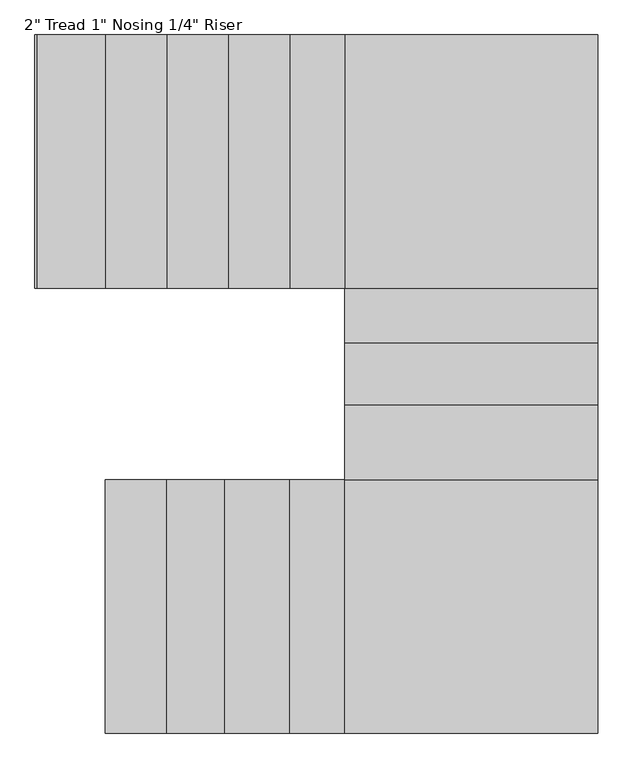
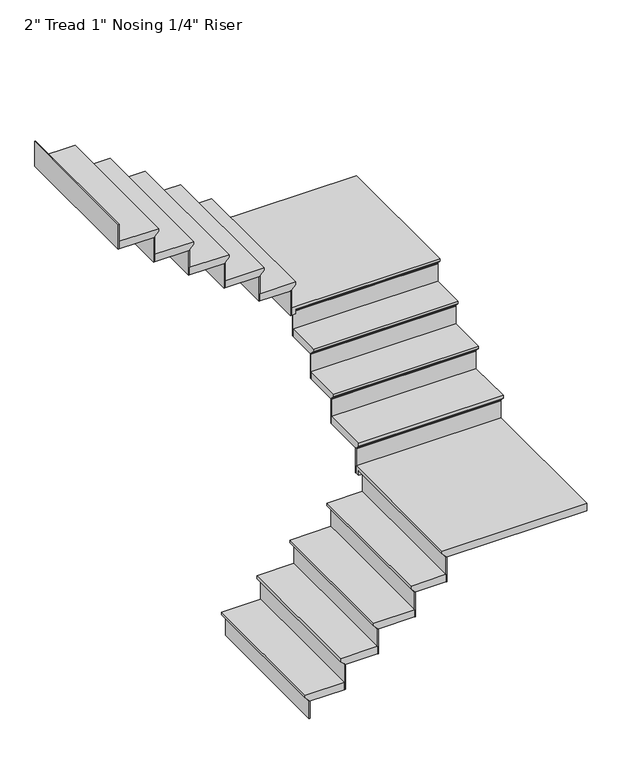
"""IFC4 building model written with IfcOpenShell, lengths in millimetres: stair flight geometry."""

from ifc_helpers import new_model, si_unit, origin, place, context, project, spatial, faceted_brep, source, transform, mapped, element, save


def stair_flight_c017ec09(model_context):
    return source(origin(), model_context, "Body", "Brep", [
        faceted_brep([(344.764115, -6141.1350571, 12951.8833333), (344.764115, -6141.1350571, 12970.9333333), (344.764115, -5201.3350571, 12970.9333333), (344.764115, -5201.3350571, 12951.8833333), (370.164115, -6141.1350571, 12926.4833333), (370.164115, -5201.3350571, 12926.4833333), (598.764115, -6141.1350571, 12970.9333333), (598.764115, -5201.3350571, 12970.9333333), (370.164115, -5201.3350571, 12920.1333333), (598.764115, -5201.3350571, 12920.1333333), (598.764115, -6141.1350571, 12920.1333333), (370.164115, -6141.1350571, 12920.1333333)], [[[0, 1, 2, 3]], [[4, 0, 3, 5]], [[2, 1, 6, 7]], [[8, 9, 10, 11]], [[2, 7, 9, 8, 5, 3]], [[8, 11, 4, 5]], [[6, 1, 0, 4, 11, 10]], [[7, 6, 10, 9]]]),
        faceted_brep([(370.164115, -6141.1350571, 12920.1333333), (370.164115, -6141.1350571, 12801.6), (376.514115, -6141.1350571, 12801.6), (376.514115, -6141.1350571, 12920.1333333), (370.164115, -5201.3350571, 12920.1333333), (376.514115, -5201.3350571, 12920.1333333), (376.514115, -5201.3350571, 12801.6), (370.164115, -5201.3350571, 12801.6)], [[[0, 1, 2, 3]], [[4, 5, 6, 7]], [[1, 0, 4, 7]], [[2, 1, 7, 6]], [[3, 2, 6, 5]], [[0, 3, 5, 4]]]),
        faceted_brep([(598.764115, -6141.1350571, 13089.4666667), (598.764115, -6141.1350571, 12920.1333333), (605.114115, -6141.1350571, 12920.1333333), (605.114115, -6141.1350571, 13089.4666667), (598.764115, -5201.3350571, 13089.4666667), (605.114115, -5201.3350571, 13089.4666667), (605.114115, -5201.3350571, 12920.1333333), (598.764115, -5201.3350571, 12920.1333333)], [[[0, 1, 2, 3]], [[4, 5, 6, 7]], [[1, 0, 4, 7]], [[2, 1, 7, 6]], [[3, 2, 6, 5]], [[0, 3, 5, 4]]]),
        faceted_brep([(573.364115, -5201.3350571, 13140.2666667), (573.364115, -6141.1350571, 13140.2666667), (814.664115, -6141.1350571, 13140.2666667), (814.664115, -5201.3350571, 13140.2666667), (598.764115, -5201.3350571, 13089.4666667), (814.664115, -5201.3350571, 13089.4666667), (814.664115, -6141.1350571, 13089.4666667), (598.764115, -6141.1350571, 13089.4666667), (598.764115, -5201.3350571, 13095.8166667), (573.364115, -5201.3350571, 13121.2166667), (598.764115, -6141.1350571, 13095.8166667), (573.364115, -6141.1350571, 13121.2166667)], [[[0, 1, 2, 3]], [[4, 5, 6, 7]], [[0, 3, 5, 4, 8, 9]], [[4, 7, 10, 8]], [[2, 1, 11, 10, 7, 6]], [[3, 2, 6, 5]], [[11, 1, 0, 9]], [[10, 11, 9, 8]]]),
        faceted_brep([(814.664115, -6141.1350571, 13258.8), (814.664115, -6141.1350571, 13089.4666667), (821.014115, -6141.1350571, 13089.4666667), (821.014115, -6141.1350571, 13258.8), (814.664115, -5201.3350571, 13258.8), (821.014115, -5201.3350571, 13258.8), (821.014115, -5201.3350571, 13089.4666667), (814.664115, -5201.3350571, 13089.4666667)], [[[0, 1, 2, 3]], [[4, 5, 6, 7]], [[1, 0, 4, 7]], [[2, 1, 7, 6]], [[3, 2, 6, 5]], [[0, 3, 5, 4]]]),
        faceted_brep([(789.264115, -5201.3350571, 13309.6), (789.264115, -6141.1350571, 13309.6), (1055.964115, -6141.1350571, 13309.6), (1055.964115, -5201.3350571, 13309.6), (814.664115, -5201.3350571, 13258.8), (1055.964115, -5201.3350571, 13258.8), (1055.964115, -6141.1350571, 13258.8), (814.664115, -6141.1350571, 13258.8), (814.664115, -5201.3350571, 13265.15), (789.264115, -5201.3350571, 13290.55), (814.664115, -6141.1350571, 13265.15), (789.264115, -6141.1350571, 13290.55)], [[[0, 1, 2, 3]], [[4, 5, 6, 7]], [[0, 3, 5, 4, 8, 9]], [[4, 7, 10, 8]], [[2, 1, 11, 10, 7, 6]], [[3, 2, 6, 5]], [[11, 1, 0, 9]], [[10, 11, 9, 8]]]),
        faceted_brep([(1055.964115, -6141.1350571, 13428.1333333), (1055.964115, -6141.1350571, 13258.8), (1062.314115, -6141.1350571, 13258.8), (1062.314115, -6141.1350571, 13428.1333333), (1055.964115, -5201.3350571, 13428.1333333), (1062.314115, -5201.3350571, 13428.1333333), (1062.314115, -5201.3350571, 13258.8), (1055.964115, -5201.3350571, 13258.8)], [[[0, 1, 2, 3]], [[4, 5, 6, 7]], [[1, 0, 4, 7]], [[2, 1, 7, 6]], [[3, 2, 6, 5]], [[0, 3, 5, 4]]]),
        faceted_brep([(1030.564115, -5201.3350571, 13478.9333333), (1030.564115, -6141.1350571, 13478.9333333), (1259.164115, -6141.1350571, 13478.9333333), (1259.164115, -5201.3350571, 13478.9333333), (1055.964115, -5201.3350571, 13428.1333333), (1259.164115, -5201.3350571, 13428.1333333), (1259.164115, -6141.1350571, 13428.1333333), (1055.964115, -6141.1350571, 13428.1333333), (1055.964115, -5201.3350571, 13434.4833333), (1030.564115, -5201.3350571, 13459.8833333), (1055.964115, -6141.1350571, 13434.4833333), (1030.564115, -6141.1350571, 13459.8833333)], [[[0, 1, 2, 3]], [[4, 5, 6, 7]], [[0, 3, 5, 4, 8, 9]], [[4, 7, 10, 8]], [[2, 1, 11, 10, 7, 6]], [[3, 2, 6, 5]], [[11, 1, 0, 9]], [[10, 11, 9, 8]]]),
        faceted_brep([(1259.164115, -6141.1350571, 13597.4666667), (1259.164115, -6141.1350571, 13428.1333333), (1265.514115, -6141.1350571, 13428.1333333), (1265.514115, -6141.1350571, 13597.4666667), (1259.164115, -5201.3350571, 13597.4666667), (1265.514115, -5201.3350571, 13597.4666667), (1265.514115, -5201.3350571, 13428.1333333), (1259.164115, -5201.3350571, 13428.1333333)], [[[0, 1, 2, 3]], [[4, 5, 6, 7]], [[1, 0, 4, 7]], [[2, 1, 7, 6]], [[3, 2, 6, 5]], [[0, 3, 5, 4]]]),
        faceted_brep([(2173.564115, -6141.1350571, 13648.2666667), (2173.564115, -5175.9350571, 13648.2666667), (1233.764115, -5175.9350571, 13648.2666667), (1233.764115, -6141.1350571, 13648.2666667), (1233.764115, -5201.3350571, 13597.4666667), (1233.764115, -5175.9350571, 13597.4666667), (2173.564115, -5175.9350571, 13597.4666667), (2173.564115, -6141.1350571, 13597.4666667), (1259.164115, -6141.1350571, 13597.4666667), (1259.164115, -5201.3350571, 13597.4666667), (1233.764115, -5201.3350571, 13629.2166667), (1233.764115, -6141.1350571, 13629.2166667), (1259.164115, -5201.3350571, 13603.8166667), (1259.164115, -6141.1350571, 13603.8166667)], [[[0, 1, 2, 3]], [[4, 5, 6, 7, 8, 9]], [[3, 2, 5, 4, 10, 11]], [[4, 9, 12, 10]], [[9, 8, 13, 12]], [[0, 3, 11, 13, 8, 7]], [[1, 0, 7, 6]], [[2, 1, 6, 5]], [[13, 11, 10, 12]]]),
        faceted_brep([(2173.564115, -5175.9350571, 13766.8), (2173.564115, -5175.9350571, 13597.4666667), (2173.564115, -5169.5850571, 13597.4666667), (2173.564115, -5169.5850571, 13766.8), (1233.764115, -5175.9350571, 13766.8), (1233.764115, -5169.5850571, 13766.8), (1233.764115, -5169.5850571, 13597.4666667), (1233.764115, -5175.9350571, 13597.4666667)], [[[0, 1, 2, 3]], [[4, 5, 6, 7]], [[1, 0, 4, 7]], [[2, 1, 7, 6]], [[3, 2, 6, 5]], [[0, 3, 5, 4]]]),
        faceted_brep([(1233.764115, -5201.3350571, 13817.6), (2173.564115, -5201.3350571, 13817.6), (2173.564115, -4896.5350571, 13817.6), (1233.764115, -4896.5350571, 13817.6), (1233.764115, -5175.9350571, 13766.8), (1233.764115, -4896.5350571, 13766.8), (2173.564115, -4896.5350571, 13766.8), (2173.564115, -5175.9350571, 13766.8), (1233.764115, -5175.9350571, 13773.15), (1233.764115, -5201.3350571, 13798.55), (2173.564115, -5175.9350571, 13773.15), (2173.564115, -5201.3350571, 13798.55)], [[[0, 1, 2, 3]], [[4, 5, 6, 7]], [[0, 3, 5, 4, 8, 9]], [[4, 7, 10, 8]], [[2, 1, 11, 10, 7, 6]], [[3, 2, 6, 5]], [[11, 1, 0, 9]], [[10, 11, 9, 8]]]),
        faceted_brep([(2173.564115, -4896.5350571, 13936.1333333), (2173.564115, -4896.5350571, 13766.8), (2173.564115, -4890.1850571, 13766.8), (2173.564115, -4890.1850571, 13936.1333333), (1233.764115, -4896.5350571, 13936.1333333), (1233.764115, -4890.1850571, 13936.1333333), (1233.764115, -4890.1850571, 13766.8), (1233.764115, -4896.5350571, 13766.8)], [[[0, 1, 2, 3]], [[4, 5, 6, 7]], [[1, 0, 4, 7]], [[2, 1, 7, 6]], [[3, 2, 6, 5]], [[0, 3, 5, 4]]]),
        faceted_brep([(1233.764115, -4921.9350571, 13986.9333333), (2173.564115, -4921.9350571, 13986.9333333), (2173.564115, -4667.9350571, 13986.9333333), (1233.764115, -4667.9350571, 13986.9333333), (1233.764115, -4896.5350571, 13936.1333333), (1233.764115, -4667.9350571, 13936.1333333), (2173.564115, -4667.9350571, 13936.1333333), (2173.564115, -4896.5350571, 13936.1333333), (1233.764115, -4896.5350571, 13942.4833333), (1233.764115, -4921.9350571, 13967.8833333), (2173.564115, -4896.5350571, 13942.4833333), (2173.564115, -4921.9350571, 13967.8833333)], [[[0, 1, 2, 3]], [[4, 5, 6, 7]], [[0, 3, 5, 4, 8, 9]], [[4, 7, 10, 8]], [[2, 1, 11, 10, 7, 6]], [[3, 2, 6, 5]], [[11, 1, 0, 9]], [[10, 11, 9, 8]]]),
        faceted_brep([(2173.564115, -4667.9350571, 14105.4666667), (2173.564115, -4667.9350571, 13936.1333333), (2173.564115, -4661.5850571, 13936.1333333), (2173.564115, -4661.5850571, 14105.4666667), (1233.764115, -4667.9350571, 14105.4666667), (1233.764115, -4661.5850571, 14105.4666667), (1233.764115, -4661.5850571, 13936.1333333), (1233.764115, -4667.9350571, 13936.1333333)], [[[0, 1, 2, 3]], [[4, 5, 6, 7]], [[1, 0, 4, 7]], [[2, 1, 7, 6]], [[3, 2, 6, 5]], [[0, 3, 5, 4]]]),
        faceted_brep([(1233.764115, -4693.3350571, 14156.2666667), (2173.564115, -4693.3350571, 14156.2666667), (2173.564115, -4464.7350571, 14156.2666667), (1233.764115, -4464.7350571, 14156.2666667), (1233.764115, -4667.9350571, 14105.4666667), (1233.764115, -4464.7350571, 14105.4666667), (2173.564115, -4464.7350571, 14105.4666667), (2173.564115, -4667.9350571, 14105.4666667), (1233.764115, -4667.9350571, 14111.8166667), (1233.764115, -4693.3350571, 14137.2166667), (2173.564115, -4667.9350571, 14111.8166667), (2173.564115, -4693.3350571, 14137.2166667)], [[[0, 1, 2, 3]], [[4, 5, 6, 7]], [[0, 3, 5, 4, 8, 9]], [[4, 7, 10, 8]], [[2, 1, 11, 10, 7, 6]], [[3, 2, 6, 5]], [[11, 1, 0, 9]], [[10, 11, 9, 8]]]),
        faceted_brep([(2173.564115, -4464.7350571, 14274.8), (2173.564115, -4464.7350571, 14105.4666667), (2173.564115, -4458.3850571, 14105.4666667), (2173.564115, -4458.3850571, 14274.8), (1233.764115, -4464.7350571, 14274.8), (1233.764115, -4458.3850571, 14274.8), (1233.764115, -4458.3850571, 14105.4666667), (1233.764115, -4464.7350571, 14105.4666667)], [[[0, 1, 2, 3]], [[4, 5, 6, 7]], [[1, 0, 4, 7]], [[2, 1, 7, 6]], [[3, 2, 6, 5]], [[0, 3, 5, 4]]]),
        faceted_brep([(2173.564115, -3550.3350571, 14325.6), (1208.364115, -3550.3350571, 14325.6), (1208.364115, -4490.1350571, 14325.6), (2173.564115, -4490.1350571, 14325.6), (1233.764115, -4490.1350571, 14274.8), (1208.364115, -4490.1350571, 14274.8), (1208.364115, -3550.3350571, 14274.8), (2173.564115, -3550.3350571, 14274.8), (2173.564115, -4464.7350571, 14274.8), (1233.764115, -4464.7350571, 14274.8), (1233.764115, -4490.1350571, 14306.55), (2173.564115, -4490.1350571, 14306.55), (1233.764115, -4464.7350571, 14281.15), (2173.564115, -4464.7350571, 14281.15)], [[[0, 1, 2, 3]], [[4, 5, 6, 7, 8, 9]], [[3, 2, 5, 4, 10, 11]], [[4, 9, 12, 10]], [[9, 8, 13, 12]], [[0, 3, 11, 13, 8, 7]], [[1, 0, 7, 6]], [[2, 1, 6, 5]], [[13, 11, 10, 12]]]),
        faceted_brep([(1208.364115, -3550.3350571, 14444.1333333), (1208.364115, -3550.3350571, 14274.8), (1202.014115, -3550.3350571, 14274.8), (1202.014115, -3550.3350571, 14444.1333333), (1208.364115, -4490.1350571, 14444.1333333), (1202.014115, -4490.1350571, 14444.1333333), (1202.014115, -4490.1350571, 14274.8), (1208.364115, -4490.1350571, 14274.8)], [[[0, 1, 2, 3]], [[4, 5, 6, 7]], [[1, 0, 4, 7]], [[2, 1, 7, 6]], [[3, 2, 6, 5]], [[0, 3, 5, 4]]]),
        faceted_brep([(1233.764115, -4490.1350571, 14494.9333333), (1233.764115, -3550.3350571, 14494.9333333), (1005.164115, -3550.3350571, 14494.9333333), (1005.164115, -4490.1350571, 14494.9333333), (1208.364115, -4490.1350571, 14444.1333333), (1005.164115, -4490.1350571, 14444.1333333), (1005.164115, -3550.3350571, 14444.1333333), (1208.364115, -3550.3350571, 14444.1333333), (1208.364115, -4490.1350571, 14450.4833333), (1233.764115, -4490.1350571, 14475.8833333), (1208.364115, -3550.3350571, 14450.4833333), (1233.764115, -3550.3350571, 14475.8833333)], [[[0, 1, 2, 3]], [[4, 5, 6, 7]], [[0, 3, 5, 4, 8, 9]], [[4, 7, 10, 8]], [[2, 1, 11, 10, 7, 6]], [[3, 2, 6, 5]], [[11, 1, 0, 9]], [[10, 11, 9, 8]]]),
        faceted_brep([(1005.164115, -3550.3350571, 14613.4666667), (1005.164115, -3550.3350571, 14444.1333333), (998.814115, -3550.3350571, 14444.1333333), (998.814115, -3550.3350571, 14613.4666667), (1005.164115, -4490.1350571, 14613.4666667), (998.814115, -4490.1350571, 14613.4666667), (998.814115, -4490.1350571, 14444.1333333), (1005.164115, -4490.1350571, 14444.1333333)], [[[0, 1, 2, 3]], [[4, 5, 6, 7]], [[1, 0, 4, 7]], [[2, 1, 7, 6]], [[3, 2, 6, 5]], [[0, 3, 5, 4]]]),
        faceted_brep([(1030.564115, -4490.1350571, 14664.2666667), (1030.564115, -3550.3350571, 14664.2666667), (776.564115, -3550.3350571, 14664.2666667), (776.564115, -4490.1350571, 14664.2666667), (1005.164115, -4490.1350571, 14613.4666667), (776.564115, -4490.1350571, 14613.4666667), (776.564115, -3550.3350571, 14613.4666667), (1005.164115, -3550.3350571, 14613.4666667), (1005.164115, -4490.1350571, 14619.8166667), (1030.564115, -4490.1350571, 14645.2166667), (1005.164115, -3550.3350571, 14619.8166667), (1030.564115, -3550.3350571, 14645.2166667)], [[[0, 1, 2, 3]], [[4, 5, 6, 7]], [[0, 3, 5, 4, 8, 9]], [[4, 7, 10, 8]], [[2, 1, 11, 10, 7, 6]], [[3, 2, 6, 5]], [[11, 1, 0, 9]], [[10, 11, 9, 8]]]),
        faceted_brep([(776.564115, -3550.3350571, 14782.8), (776.564115, -3550.3350571, 14613.4666667), (770.214115, -3550.3350571, 14613.4666667), (770.214115, -3550.3350571, 14782.8), (776.564115, -4490.1350571, 14782.8), (770.214115, -4490.1350571, 14782.8), (770.214115, -4490.1350571, 14613.4666667), (776.564115, -4490.1350571, 14613.4666667)], [[[0, 1, 2, 3]], [[4, 5, 6, 7]], [[1, 0, 4, 7]], [[2, 1, 7, 6]], [[3, 2, 6, 5]], [[0, 3, 5, 4]]]),
        faceted_brep([(801.964115, -4490.1350571, 14833.6), (801.964115, -3550.3350571, 14833.6), (547.964115, -3550.3350571, 14833.6), (547.964115, -4490.1350571, 14833.6), (776.564115, -4490.1350571, 14782.8), (547.964115, -4490.1350571, 14782.8), (547.964115, -3550.3350571, 14782.8), (776.564115, -3550.3350571, 14782.8), (776.564115, -4490.1350571, 14789.15), (801.964115, -4490.1350571, 14814.55), (776.564115, -3550.3350571, 14789.15), (801.964115, -3550.3350571, 14814.55)], [[[0, 1, 2, 3]], [[4, 5, 6, 7]], [[0, 3, 5, 4, 8, 9]], [[4, 7, 10, 8]], [[2, 1, 11, 10, 7, 6]], [[3, 2, 6, 5]], [[11, 1, 0, 9]], [[10, 11, 9, 8]]]),
        faceted_brep([(547.964115, -3550.3350571, 14952.1333333), (547.964115, -3550.3350571, 14782.8), (541.614115, -3550.3350571, 14782.8), (541.614115, -3550.3350571, 14952.1333333), (547.964115, -4490.1350571, 14952.1333333), (541.614115, -4490.1350571, 14952.1333333), (541.614115, -4490.1350571, 14782.8), (547.964115, -4490.1350571, 14782.8)], [[[0, 1, 2, 3]], [[4, 5, 6, 7]], [[1, 0, 4, 7]], [[2, 1, 7, 6]], [[3, 2, 6, 5]], [[0, 3, 5, 4]]]),
        faceted_brep([(573.364115, -4490.1350571, 15002.9333333), (573.364115, -3550.3350571, 15002.9333333), (319.364115, -3550.3350571, 15002.9333333), (319.364115, -4490.1350571, 15002.9333333), (547.964115, -4490.1350571, 14952.1333333), (319.364115, -4490.1350571, 14952.1333333), (319.364115, -3550.3350571, 14952.1333333), (547.964115, -3550.3350571, 14952.1333333), (547.964115, -4490.1350571, 14958.4833333), (573.364115, -4490.1350571, 14983.8833333), (547.964115, -3550.3350571, 14958.4833333), (573.364115, -3550.3350571, 14983.8833333)], [[[0, 1, 2, 3]], [[4, 5, 6, 7]], [[0, 3, 5, 4, 8, 9]], [[4, 7, 10, 8]], [[2, 1, 11, 10, 7, 6]], [[3, 2, 6, 5]], [[11, 1, 0, 9]], [[10, 11, 9, 8]]]),
        faceted_brep([(319.364115, -3550.3350571, 15121.4666667), (319.364115, -3550.3350571, 14952.1333333), (313.014115, -3550.3350571, 14952.1333333), (313.014115, -3550.3350571, 15121.4666667), (319.364115, -4490.1350571, 15121.4666667), (313.014115, -4490.1350571, 15121.4666667), (313.014115, -4490.1350571, 14952.1333333), (319.364115, -4490.1350571, 14952.1333333)], [[[0, 1, 2, 3]], [[4, 5, 6, 7]], [[1, 0, 4, 7]], [[2, 1, 7, 6]], [[3, 2, 6, 5]], [[0, 3, 5, 4]]]),
        faceted_brep([(90.764115, -3550.3350571, 15290.8), (90.764115, -3550.3350571, 15121.4666667), (84.414115, -3550.3350571, 15121.4666667), (84.414115, -3550.3350571, 15290.8), (90.764115, -4490.1350571, 15290.8), (84.414115, -4490.1350571, 15290.8), (84.414115, -4490.1350571, 15121.4666667), (90.764115, -4490.1350571, 15121.4666667)], [[[0, 1, 2, 3]], [[4, 5, 6, 7]], [[1, 0, 4, 7]], [[2, 1, 7, 6]], [[3, 2, 6, 5]], [[0, 3, 5, 4]]]),
        faceted_brep([(344.764115, -4490.1350571, 15172.2666667), (344.764115, -3550.3350571, 15172.2666667), (90.764115, -3550.3350571, 15172.2666667), (90.764115, -4490.1350571, 15172.2666667), (319.364115, -4490.1350571, 15121.4666667), (90.764115, -4490.1350571, 15121.4666667), (90.764115, -3550.3350571, 15121.4666667), (319.364115, -3550.3350571, 15121.4666667), (319.364115, -4490.1350571, 15127.8166667), (344.764115, -4490.1350571, 15153.2166667), (319.364115, -3550.3350571, 15127.8166667), (344.764115, -3550.3350571, 15153.2166667)], [[[0, 1, 2, 3]], [[4, 5, 6, 7]], [[0, 3, 5, 4, 8, 9]], [[4, 7, 10, 8]], [[2, 1, 11, 10, 7, 6]], [[3, 2, 6, 5]], [[11, 1, 0, 9]], [[10, 11, 9, 8]]]),
    ])


if __name__ == "__main__":
    model = new_model("IFC4")
    model_context = context("Model", 3, world=origin())
    ifc_project = project(units=[si_unit("LENGTHUNIT", "METRE", prefix="MILLI")], contexts=[model_context])
    site = spatial("IfcSite", under=ifc_project)
    building = spatial("IfcBuilding", under=site)
    placement = place(None, origin())
    stair_flight_shape = stair_flight_c017ec09(model_context)
    element("IfcStairFlight", 1, ObjectType="2\" Tread 1\" Nosing 1/4\" Riser", at=placement, inside=building, context=model_context, shape_type="MappedRepresentation", body=[
        mapped(stair_flight_shape, transform((0.0, 0.0, 0.0), x_axis=(1.0, 0.0, 0.0), y_axis=(0.0, 1.0, 0.0), z_axis=(0.0, 0.0, 1.0))),
    ])
    save(model, "model.ifc")
